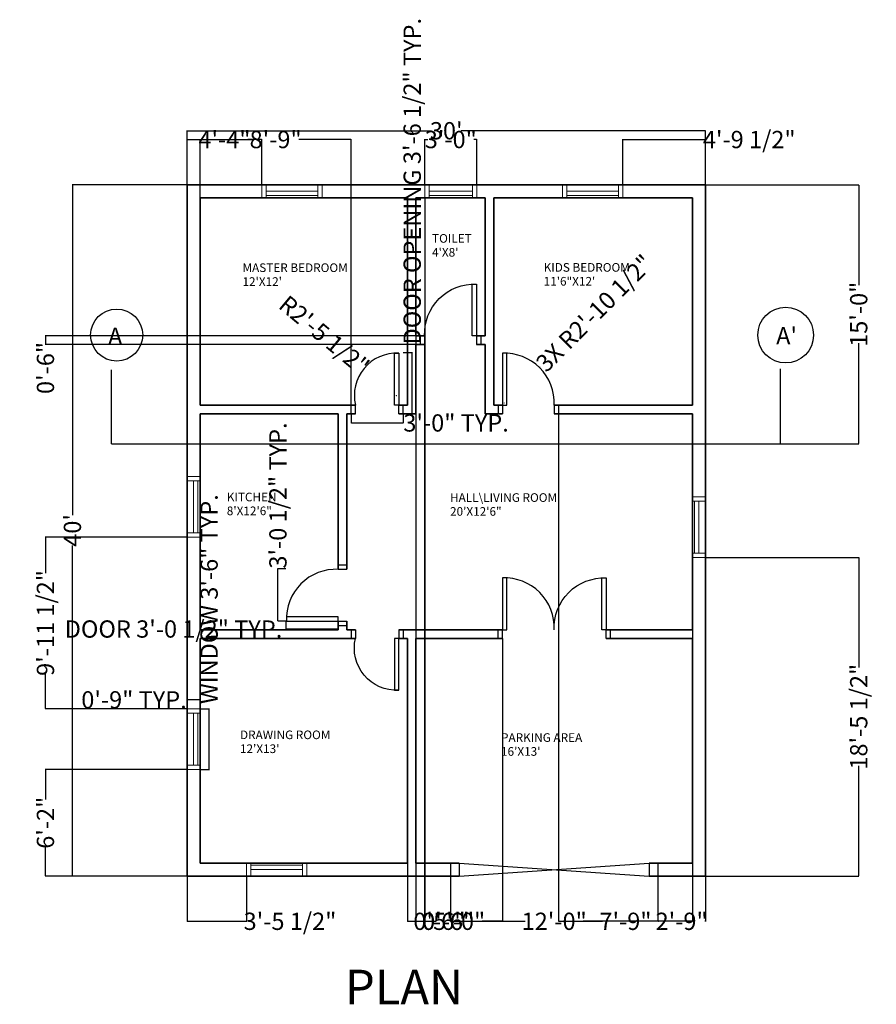
# Model space of a CAD drawing. Units: inches. Extents: x -91 to 1027, y -85 to 599.
# Tile 1 of 3: x -91 to 504, y -85 to 599. Entities that reach past the tile are written whole.
import ezdxf

# ---------------------------------------------------------------- set-up
doc = ezdxf.new("R2010")
doc.units = ezdxf.units.IN
doc.header["$MEASUREMENT"] = 0
for name, color, linetype, lineweight in [('A-ANNO-DIMS', 2, 'Continuous', 18), ('A-ANNO-SYMB', 1, 'Continuous', 25), ('A-ANNO-TEXT', 7, 'Continuous', 35), ('A-AREA-IDEN', 7, 'Continuous', 18), ('A-DOOR', 3, 'Continuous', 25), ('A-DOOR-GATE', 3, 'Continuous', 25), ('A-GLAZ', 4, 'Continuous', 18), ('A-WALL', 7, 'Continuous', 35)]:
    doc.layers.add(name, color=color, linetype=linetype, lineweight=lineweight)
doc.styles.get("Standard").update_dxf_attribs({"font": 'arial.ttf'})
doc.dimstyles.get("Standard").update_dxf_attribs({"dimtxt": 12, "dimasz": 0.18, "dimexe": 0.18, "dimexo": 0.0625, "dimgap": 0.09, "dimtad": 0, "dimdec": 1, "dimzin": 0, "dimdsep": 46, "dimlunit": 3, "dimtxsty": 'Standard', "dimcen": 0.09, "dimadec": 0, "dimazin": 0, "dimtfac": 1, "dimtdec": 1, "dimtofl": 0, "dimtmove": 0, "dimatfit": 3, "dimfxl": 1, "dimtolj": 1, "dimtzin": 0, "dimarcsym": 0})

# ---------------------------------------------------------------- blocks, each defined once
blk = doc.blocks.new('*D1')
at = {"layer": 'A-ANNO-DIMS', "color": 0, "lineweight": -2, "transparency": 16777216}
for p, q in [((25.15, 484.59), (25.15, 522.21)), ((25.33, 522.03), (194.88, 522.03)), ((384.97, 522.03), (215.41, 522.03)), ((385.15, 484.59), (385.15, 522.21))]:
    blk.add_line(p, q, dxfattribs=at)
at = {"layer": 'A-ANNO-DIMS', "color": 0, "transparency": 16777216}
for points in [[(25.33, 522.06), (25.33, 522), (25.15, 522.03)], [(384.97, 522.06), (384.97, 522), (385.15, 522.03)]]:
    blk.add_solid(points, dxfattribs=at)
at = {"layer": 'Defpoints', "color": 0, "transparency": 16777216}
for p in [(385.15, 522.03), (25.15, 484.52), (385.15, 484.52)]:
    blk.add_point(p, dxfattribs=at)
at = {"layer": 'A-ANNO-DIMS', "color": 0, "transparency": 16777216, "insert": (205.15, 522.03), "char_height": 12, "attachment_point": 5}
blk.add_mtext("\\A1;30'", dxfattribs=at)
blk = doc.blocks.new('*D2')
at = {"layer": 'A-ANNO-DIMS', "color": 0, "lineweight": -2, "transparency": 16777216}
for p, q in [((25.08, 484.52), (-54.67, 484.52)), ((-54.49, 484.34), (-54.49, 255.04)), ((-54.49, 4.7), (-54.49, 234.01)), ((25.08, 4.52), (-54.67, 4.52))]:
    blk.add_line(p, q, dxfattribs=at)
at = {"layer": 'A-ANNO-DIMS', "color": 0, "transparency": 16777216}
for points in [[(-54.52, 484.34), (-54.46, 484.34), (-54.49, 484.52)], [(-54.52, 4.7), (-54.46, 4.7), (-54.49, 4.52)]]:
    blk.add_solid(points, dxfattribs=at)
at = {"layer": 'Defpoints', "color": 0, "transparency": 16777216}
for p in [(-54.49, 484.52), (25.15, 484.52), (25.15, 4.52)]:
    blk.add_point(p, dxfattribs=at)
at = {"layer": 'A-ANNO-DIMS', "color": 0, "transparency": 16777216, "insert": (-54.49, 244.52), "char_height": 12, "attachment_point": 5, "rotation": 90}
blk.add_mtext("\\A1;40'", dxfattribs=at)
blk = doc.blocks.new('WIN-36-PLAN')
for p, q in [((0, 9), (0, 0)), ((39, 9), (3, 9)), ((3, 9), (3, 0)), ((39, 0), (39, 9)), ((42, 0), (42, 9)), ((3, 4.5), (39, 4.5)), ((3, 1.5), (39, 1.5)), ((3, 0), (39, 0))]:
    blk.add_line(p, q)
blk = doc.blocks.new('DOOR-36-PLAN')
blk.add_lwpolyline([(0, 0), (3, 0), (3, 36), (0, 36)], close=True)
blk.add_arc((1.5, 1.5), 34.53, 357.51045, 92.48955)
blk = doc.blocks.new('DOOR-30-OPENING-PLAN')
for p, q in [((0, 0), (0, 6)), ((3, 0), (3, 6)), ((33, 0), (33, 6)), ((36, 0), (36, 6))]:
    blk.add_line(p, q)
blk.add_lwpolyline([(33, 6), (30, 6), (30, 42), (33, 42)], close=True)
blk.add_arc((31.5, 12.75), 29.29, 87.06433, 193.32453)
blk = doc.blocks.new('*D24')
at = {"layer": 'A-ANNO-DIMS', "color": 0, "lineweight": -2, "transparency": 16777216}
for p, q in [((34.21, 120.6), (40.63, 120.6)), ((40.45, 120.6), (40.45, 120.78)), ((40.45, 78.78), (40.45, 120.42)), ((34.21, 78.6), (40.63, 78.6))]:
    blk.add_line(p, q, dxfattribs=at)
at = {"layer": 'A-ANNO-DIMS', "color": 0, "transparency": 16777216}
for points in [[(40.42, 120.42), (40.48, 120.42), (40.45, 120.6)], [(40.42, 78.78), (40.48, 78.78), (40.45, 78.6)]]:
    blk.add_solid(points, dxfattribs=at)
at = {"layer": 'Defpoints', "color": 0, "transparency": 16777216}
for p in [(34.15, 120.6), (40.45, 120.6), (34.15, 78.6)]:
    blk.add_point(p, dxfattribs=at)
at = {"layer": 'A-ANNO-DIMS', "color": 0, "transparency": 16777216, "insert": (40.45, 196.8), "char_height": 12, "attachment_point": 5, "rotation": 90}
blk.add_mtext('\\A1;WINDOW 3\'-6" TYP.', dxfattribs=at)
blk = doc.blocks.new('*D25')
at = {"layer": 'A-ANNO-DIMS', "color": 0, "lineweight": -2, "transparency": 16777216}
for p, q in [((25.15, 126.9), (24.97, 126.9)), ((25.15, 120.67), (25.15, 127.08)), ((33.97, 126.9), (25.33, 126.9)), ((34.15, 120.67), (34.15, 127.08))]:
    blk.add_line(p, q, dxfattribs=at)
at = {"layer": 'A-ANNO-DIMS', "color": 0, "transparency": 16777216}
for points in [[(25.33, 126.93), (25.33, 126.87), (25.15, 126.9)], [(33.97, 126.93), (33.97, 126.87), (34.15, 126.9)]]:
    blk.add_solid(points, dxfattribs=at)
at = {"layer": 'Defpoints', "color": 0, "transparency": 16777216}
for p in [(25.15, 126.9), (25.15, 120.6), (34.15, 120.6)]:
    blk.add_point(p, dxfattribs=at)
at = {"layer": 'A-ANNO-DIMS', "color": 0, "transparency": 16777216, "insert": (-11.7, 126.9), "char_height": 12, "attachment_point": 5}
blk.add_mtext('\\A1;0\'-9" TYP.', dxfattribs=at)
blk = doc.blocks.new('*D26')
at = {"layer": 'A-ANNO-DIMS', "color": 0, "lineweight": -2, "transparency": 16777216}
for p, q in [((93.73, 181.46), (93.73, 175.88)), ((130.15, 181.46), (130.15, 175.88)), ((93.73, 176.06), (93.55, 176.06)), ((129.97, 176.06), (93.91, 176.06))]:
    blk.add_line(p, q, dxfattribs=at)
at = {"layer": 'A-ANNO-DIMS', "color": 0, "transparency": 16777216}
for points in [[(93.91, 176.09), (93.91, 176.03), (93.73, 176.06)], [(129.97, 176.09), (129.97, 176.03), (130.15, 176.06)]]:
    blk.add_solid(points, dxfattribs=at)
at = {"layer": 'Defpoints', "color": 0, "transparency": 16777216}
for p in [(93.73, 181.52), (130.15, 181.52), (93.73, 176.06)]:
    blk.add_point(p, dxfattribs=at)
at = {"layer": 'A-ANNO-DIMS', "color": 0, "transparency": 16777216, "insert": (15.73, 176.06), "char_height": 12, "attachment_point": 5}
blk.add_mtext('\\A1;DOOR 3\'-0 1/2" TYP.', dxfattribs=at)
blk = doc.blocks.new('*D27')
at = {"layer": 'A-ANNO-DIMS', "color": 0, "lineweight": -2, "transparency": 16777216}
for p, q in [((93.66, 217.94), (88.08, 217.94)), ((88.26, 217.94), (88.26, 218.12)), ((88.26, 181.7), (88.26, 217.76)), ((93.66, 181.52), (88.08, 181.52))]:
    blk.add_line(p, q, dxfattribs=at)
at = {"layer": 'A-ANNO-DIMS', "color": 0, "transparency": 16777216}
for points in [[(88.23, 217.76), (88.29, 217.76), (88.26, 217.94)], [(88.23, 181.7), (88.29, 181.7), (88.26, 181.52)]]:
    blk.add_solid(points, dxfattribs=at)
at = {"layer": 'Defpoints', "color": 0, "transparency": 16777216}
for p in [(88.26, 217.94), (93.73, 217.94), (93.73, 181.52)]:
    blk.add_point(p, dxfattribs=at)
at = {"layer": 'A-ANNO-DIMS', "color": 0, "transparency": 16777216, "insert": (88.26, 268.76), "char_height": 12, "attachment_point": 5, "rotation": 90}
blk.add_mtext('\\A1;3\'-0 1/2" TYP.', dxfattribs=at)
blk = doc.blocks.new('*D28')
at = {"layer": 'A-ANNO-DIMS', "color": 0, "lineweight": -2, "transparency": 16777216}
for p, q in [((175.21, 368), (181.7, 368)), ((181.52, 368), (181.52, 368.18)), ((181.52, 325.7), (181.52, 367.82)), ((175.21, 325.52), (181.7, 325.52))]:
    blk.add_line(p, q, dxfattribs=at)
at = {"layer": 'A-ANNO-DIMS', "color": 0, "transparency": 16777216}
for points in [[(181.49, 367.82), (181.55, 367.82), (181.52, 368)], [(181.49, 325.7), (181.55, 325.7), (181.52, 325.52)]]:
    blk.add_solid(points, dxfattribs=at)
at = {"layer": 'Defpoints', "color": 0, "transparency": 16777216}
for p in [(175.15, 368), (181.52, 368), (175.15, 325.52)]:
    blk.add_point(p, dxfattribs=at)
at = {"layer": 'A-ANNO-DIMS', "color": 0, "transparency": 16777216, "insert": (181.52, 486.98), "char_height": 12, "attachment_point": 5, "rotation": 90}
blk.add_mtext('\\A1;DOOR OPENING 3\'-6 1/2" TYP.', dxfattribs=at)
blk = doc.blocks.new('*D29')
at = {"layer": 'A-ANNO-DIMS', "color": 0, "lineweight": -2, "transparency": 16777216}
for p, q in [((139.15, 325.46), (139.15, 318.97)), ((175.15, 325.46), (175.15, 318.97)), ((139.33, 319.15), (174.97, 319.15)), ((175.15, 319.15), (175.33, 319.15))]:
    blk.add_line(p, q, dxfattribs=at)
at = {"layer": 'A-ANNO-DIMS', "color": 0, "transparency": 16777216}
for points in [[(139.33, 319.18), (139.33, 319.12), (139.15, 319.15)], [(174.97, 319.18), (174.97, 319.12), (175.15, 319.15)]]:
    blk.add_solid(points, dxfattribs=at)
at = {"layer": 'Defpoints', "color": 0, "transparency": 16777216}
for p in [(139.15, 325.52), (175.15, 325.52), (175.15, 319.15)]:
    blk.add_point(p, dxfattribs=at)
at = {"layer": 'A-ANNO-DIMS', "color": 0, "transparency": 16777216, "insert": (211.98, 319.15), "char_height": 12, "attachment_point": 5}
blk.add_mtext('\\A1;3\'-0" TYP.', dxfattribs=at)
blk = doc.blocks.new('*D36')
at = {"layer": 'A-ANNO-DIMS', "color": 0, "lineweight": -2, "transparency": 16777216}
for p, q in [((25.15, 484.59), (25.15, 516.1)), ((25.33, 515.92), (34.83, 515.92)), ((76.89, 515.92), (67.39, 515.92)), ((77.07, 484.59), (77.07, 516.1))]:
    blk.add_line(p, q, dxfattribs=at)
at = {"layer": 'A-ANNO-DIMS', "color": 0, "transparency": 16777216}
for points in [[(25.33, 515.95), (25.33, 515.89), (25.15, 515.92)], [(76.89, 515.95), (76.89, 515.89), (77.07, 515.92)]]:
    blk.add_solid(points, dxfattribs=at)
at = {"layer": 'Defpoints', "color": 0, "transparency": 16777216}
for p in [(77.07, 515.92), (25.15, 484.52), (77.07, 484.52)]:
    blk.add_point(p, dxfattribs=at)
at = {"layer": 'A-ANNO-DIMS', "color": 0, "transparency": 16777216, "insert": (51.11, 515.92), "char_height": 12, "attachment_point": 5}
blk.add_mtext('\\A1;4\'-4"', dxfattribs=at)
blk = doc.blocks.new('*D37')
at = {"layer": 'A-ANNO-DIMS', "color": 0, "lineweight": -2, "transparency": 16777216}
for p, q in [((184.15, 475.46), (184.15, -27.06)), ((190.32, 475.46), (190.32, -27.06)), ((184.33, -26.88), (190.14, -26.88)), ((190.32, -26.88), (190.5, -26.88))]:
    blk.add_line(p, q, dxfattribs=at)
at = {"layer": 'A-ANNO-DIMS', "color": 0, "transparency": 16777216}
for points in [[(184.33, -26.85), (184.33, -26.91), (184.15, -26.88)], [(190.14, -26.85), (190.14, -26.91), (190.32, -26.88)]]:
    blk.add_solid(points, dxfattribs=at)
at = {"layer": 'Defpoints', "color": 0, "transparency": 16777216}
for p in [(184.15, 475.52), (190.32, 475.52), (190.32, -26.88)]:
    blk.add_point(p, dxfattribs=at)
at = {"layer": 'A-ANNO-DIMS', "color": 0, "transparency": 16777216, "insert": (206.54, -26.88), "char_height": 12, "attachment_point": 5}
blk.add_mtext('\\A1;0\'-6"', dxfattribs=at)
blk = doc.blocks.new('*D38')
at = {"layer": 'A-ANNO-DIMS', "color": 0, "lineweight": -2, "transparency": 16777216}
for p, q in [((190.32, 484.59), (190.32, 516.1)), ((190.5, 515.92), (192.29, 515.92)), ((226.14, 515.92), (224.36, 515.92)), ((226.32, 484.59), (226.32, 516.1))]:
    blk.add_line(p, q, dxfattribs=at)
at = {"layer": 'A-ANNO-DIMS', "color": 0, "transparency": 16777216}
for points in [[(190.5, 515.95), (190.5, 515.89), (190.32, 515.92)], [(226.14, 515.95), (226.14, 515.89), (226.32, 515.92)]]:
    blk.add_solid(points, dxfattribs=at)
at = {"layer": 'Defpoints', "color": 0, "transparency": 16777216}
for p in [(226.32, 515.92), (190.32, 484.52), (226.32, 484.52)]:
    blk.add_point(p, dxfattribs=at)
at = {"layer": 'A-ANNO-DIMS', "color": 0, "transparency": 16777216, "insert": (208.32, 515.92), "char_height": 12, "attachment_point": 5}
blk.add_mtext('\\A1;3\'-0"', dxfattribs=at)
blk = doc.blocks.new('*D39')
at = {"layer": 'A-ANNO-DIMS', "color": 0, "lineweight": -2, "transparency": 16777216}
for p, q in [((327.88, 484.59), (327.88, 516.1)), ((328.06, 515.92), (384.97, 515.92)), ((385.15, 484.59), (385.15, 516.1)), ((385.15, 515.92), (385.33, 515.92))]:
    blk.add_line(p, q, dxfattribs=at)
at = {"layer": 'A-ANNO-DIMS', "color": 0, "transparency": 16777216}
for points in [[(328.06, 515.95), (328.06, 515.89), (327.88, 515.92)], [(384.97, 515.95), (384.97, 515.89), (385.15, 515.92)]]:
    blk.add_solid(points, dxfattribs=at)
at = {"layer": 'Defpoints', "color": 0, "transparency": 16777216}
for p in [(385.15, 515.92), (327.88, 484.52), (385.15, 484.52)]:
    blk.add_point(p, dxfattribs=at)
at = {"layer": 'A-ANNO-DIMS', "color": 0, "transparency": 16777216, "insert": (415.59, 515.92), "char_height": 12, "attachment_point": 5}
blk.add_mtext('\\A1;4\'-9 1/2"', dxfattribs=at)
blk = doc.blocks.new('*D40')
at = {"layer": 'A-ANNO-DIMS', "color": 0, "lineweight": -2, "transparency": 16777216}
for p, q in [((25.15, 4.46), (25.15, -27.06)), ((66.43, 4.46), (66.43, -27.06)), ((25.33, -26.88), (66.25, -26.88)), ((66.43, -26.88), (66.61, -26.88))]:
    blk.add_line(p, q, dxfattribs=at)
at = {"layer": 'A-ANNO-DIMS', "color": 0, "transparency": 16777216}
for points in [[(25.33, -26.85), (25.33, -26.91), (25.15, -26.88)], [(66.25, -26.85), (66.25, -26.91), (66.43, -26.88)]]:
    blk.add_solid(points, dxfattribs=at)
at = {"layer": 'Defpoints', "color": 0, "transparency": 16777216}
for p in [(25.15, 4.52), (66.43, 4.52), (66.43, -26.88)]:
    blk.add_point(p, dxfattribs=at)
at = {"layer": 'A-ANNO-DIMS', "color": 0, "transparency": 16777216, "insert": (96.63, -26.88), "char_height": 12, "attachment_point": 5}
blk.add_mtext('\\A1;3\'-5 1/2"', dxfattribs=at)
blk = doc.blocks.new('*D41')
at = {"layer": 'A-ANNO-DIMS', "color": 0, "lineweight": -2, "transparency": 16777216}
for p, q in [((352.15, 4.46), (352.15, -27.06)), ((385.15, 4.46), (385.15, -27.06)), ((352.33, -26.88), (352.5, -26.88)), ((384.97, -26.88), (384.79, -26.88))]:
    blk.add_line(p, q, dxfattribs=at)
at = {"layer": 'A-ANNO-DIMS', "color": 0, "transparency": 16777216}
for points in [[(352.33, -26.85), (352.33, -26.91), (352.15, -26.88)], [(384.97, -26.85), (384.97, -26.91), (385.15, -26.88)]]:
    blk.add_solid(points, dxfattribs=at)
at = {"layer": 'Defpoints', "color": 0, "transparency": 16777216}
for p in [(352.15, 4.52), (385.15, 4.52), (352.15, -26.88)]:
    blk.add_point(p, dxfattribs=at)
at = {"layer": 'A-ANNO-DIMS', "color": 0, "transparency": 16777216, "insert": (368.65, -26.88), "char_height": 12, "attachment_point": 5}
blk.add_mtext('\\A1;2\'-9"', dxfattribs=at)
blk = doc.blocks.new('*D42')
at = {"layer": 'A-ANNO-DIMS', "color": 0, "lineweight": -2, "transparency": 16777216}
for p, q in [((208.15, 4.46), (208.15, -27.06)), ((352.15, 4.46), (352.15, -27.06)), ((208.33, -26.88), (260.01, -26.88)), ((351.97, -26.88), (300.28, -26.88))]:
    blk.add_line(p, q, dxfattribs=at)
at = {"layer": 'A-ANNO-DIMS', "color": 0, "transparency": 16777216}
for points in [[(208.33, -26.85), (208.33, -26.91), (208.15, -26.88)], [(351.97, -26.85), (351.97, -26.91), (352.15, -26.88)]]:
    blk.add_solid(points, dxfattribs=at)
at = {"layer": 'Defpoints', "color": 0, "transparency": 16777216}
for p in [(208.15, 4.52), (352.15, 4.52), (352.15, -26.88)]:
    blk.add_point(p, dxfattribs=at)
at = {"layer": 'A-ANNO-DIMS', "color": 0, "transparency": 16777216, "insert": (280.15, -26.88), "char_height": 12, "attachment_point": 5}
blk.add_mtext('\\A1;12\'-0"', dxfattribs=at)
blk = doc.blocks.new('*D43')
at = {"layer": 'A-ANNO-DIMS', "color": 0, "lineweight": -2, "transparency": 16777216}
for p, q in [((25.08, 78.6), (-73.39, 78.6)), ((-73.21, 78.42), (-73.21, 57.64)), ((-73.21, 4.7), (-73.21, 25.49)), ((25.08, 4.52), (-73.39, 4.52))]:
    blk.add_line(p, q, dxfattribs=at)
at = {"layer": 'A-ANNO-DIMS', "color": 0, "transparency": 16777216}
for points in [[(-73.24, 78.42), (-73.18, 78.42), (-73.21, 78.6)], [(-73.24, 4.7), (-73.18, 4.7), (-73.21, 4.52)]]:
    blk.add_solid(points, dxfattribs=at)
at = {"layer": 'Defpoints', "color": 0, "transparency": 16777216}
for p in [(-73.21, 78.6), (25.15, 78.6), (25.15, 4.52)]:
    blk.add_point(p, dxfattribs=at)
at = {"layer": 'A-ANNO-DIMS', "color": 0, "transparency": 16777216, "insert": (-73.21, 41.56), "char_height": 12, "attachment_point": 5, "rotation": 90}
blk.add_mtext('\\A1;6\'-2"', dxfattribs=at)
blk = doc.blocks.new('*D44')
at = {"layer": 'A-ANNO-DIMS', "color": 0, "lineweight": -2, "transparency": 16777216}
for p, q in [((25.08, 239.92), (-73.39, 239.92)), ((-73.21, 239.74), (-73.21, 214.95)), ((-73.21, 120.78), (-73.21, 145.58)), ((25.08, 120.6), (-73.39, 120.6))]:
    blk.add_line(p, q, dxfattribs=at)
at = {"layer": 'A-ANNO-DIMS', "color": 0, "transparency": 16777216}
for points in [[(-73.24, 239.74), (-73.18, 239.74), (-73.21, 239.92)], [(-73.24, 120.78), (-73.18, 120.78), (-73.21, 120.6)]]:
    blk.add_solid(points, dxfattribs=at)
at = {"layer": 'Defpoints', "color": 0, "transparency": 16777216}
for p in [(25.15, 239.92), (-73.21, 120.6), (25.15, 120.6)]:
    blk.add_point(p, dxfattribs=at)
at = {"layer": 'A-ANNO-DIMS', "color": 0, "transparency": 16777216, "insert": (-73.21, 180.26), "char_height": 12, "attachment_point": 5, "rotation": 90}
blk.add_mtext('\\A1;9\'-11 1/2"', dxfattribs=at)
blk = doc.blocks.new('*D45')
at = {"layer": 'A-ANNO-DIMS', "color": 0, "lineweight": -2, "transparency": 16777216}
for p, q in [((385.21, 225.81), (491.83, 225.81)), ((491.65, 225.63), (491.65, 149.28)), ((491.65, 4.7), (491.65, 81.05)), ((385.21, 4.52), (491.83, 4.52))]:
    blk.add_line(p, q, dxfattribs=at)
at = {"layer": 'A-ANNO-DIMS', "color": 0, "transparency": 16777216}
for points in [[(491.62, 225.63), (491.68, 225.63), (491.65, 225.81)], [(491.62, 4.7), (491.68, 4.7), (491.65, 4.52)]]:
    blk.add_solid(points, dxfattribs=at)
at = {"layer": 'Defpoints', "color": 0, "transparency": 16777216}
for p in [(385.15, 225.81), (491.65, 225.81), (385.15, 4.52)]:
    blk.add_point(p, dxfattribs=at)
at = {"layer": 'A-ANNO-DIMS', "color": 0, "transparency": 16777216, "insert": (491.65, 115.17), "char_height": 12, "attachment_point": 5, "rotation": 90}
blk.add_mtext('\\A1;18\'-5 1/2"', dxfattribs=at)
blk = doc.blocks.new('*D46')
at = {"layer": 'A-ANNO-DIMS', "color": 0, "lineweight": -2, "transparency": 16777216}
for p, q in [((178.15, 13.46), (178.15, -27.06)), ((184.15, 13.46), (184.15, -27.06)), ((178.33, -26.88), (183.97, -26.88)), ((184.15, -26.88), (184.33, -26.88))]:
    blk.add_line(p, q, dxfattribs=at)
at = {"layer": 'A-ANNO-DIMS', "color": 0, "transparency": 16777216}
for points in [[(178.33, -26.85), (178.33, -26.91), (178.15, -26.88)], [(183.97, -26.85), (183.97, -26.91), (184.15, -26.88)]]:
    blk.add_solid(points, dxfattribs=at)
at = {"layer": 'Defpoints', "color": 0, "transparency": 16777216}
for p in [(178.15, 13.52), (184.15, 13.52), (184.15, -26.88)]:
    blk.add_point(p, dxfattribs=at)
at = {"layer": 'A-ANNO-DIMS', "color": 0, "transparency": 16777216, "insert": (200.37, -26.88), "char_height": 12, "attachment_point": 5}
blk.add_mtext('\\A1;0\'-6"', dxfattribs=at)
blk = doc.blocks.new('*D47')
at = {"layer": 'A-ANNO-DIMS', "color": 0, "lineweight": -2, "transparency": 16777216}
for p, q in [((385.21, 484.52), (491.83, 484.52)), ((491.65, 484.34), (491.65, 414.74)), ((491.65, 304.87), (491.65, 374.47)), ((437.43, 304.69), (491.83, 304.69))]:
    blk.add_line(p, q, dxfattribs=at)
at = {"layer": 'A-ANNO-DIMS', "color": 0, "transparency": 16777216}
for points in [[(491.62, 484.34), (491.68, 484.34), (491.65, 484.52)], [(491.62, 304.87), (491.68, 304.87), (491.65, 304.69)]]:
    blk.add_solid(points, dxfattribs=at)
at = {"layer": 'Defpoints', "color": 0, "transparency": 16777216}
for p in [(385.15, 484.52), (491.65, 484.52), (437.37, 304.69)]:
    blk.add_point(p, dxfattribs=at)
at = {"layer": 'A-ANNO-DIMS', "color": 0, "transparency": 16777216, "insert": (491.65, 394.6), "char_height": 12, "attachment_point": 5, "rotation": 90}
blk.add_mtext('\\A1;15\'-0"', dxfattribs=at)
blk = doc.blocks.new('*D48')
at = {"layer": 'A-ANNO-DIMS', "color": 0, "lineweight": -2, "transparency": 16777216}
for p, q in [((184.15, 169.46), (184.15, -27.06)), ((244.15, 169.46), (244.15, -27.06)), ((184.33, -26.88), (198.11, -26.88)), ((243.97, -26.88), (230.19, -26.88))]:
    blk.add_line(p, q, dxfattribs=at)
at = {"layer": 'A-ANNO-DIMS', "color": 0, "transparency": 16777216}
for points in [[(184.33, -26.85), (184.33, -26.91), (184.15, -26.88)], [(243.97, -26.85), (243.97, -26.91), (244.15, -26.88)]]:
    blk.add_solid(points, dxfattribs=at)
at = {"layer": 'Defpoints', "color": 0, "transparency": 16777216}
for p in [(184.15, 169.52), (244.15, 169.52), (244.15, -26.88)]:
    blk.add_point(p, dxfattribs=at)
at = {"layer": 'A-ANNO-DIMS', "color": 0, "transparency": 16777216, "insert": (214.15, -26.88), "char_height": 12, "attachment_point": 5}
blk.add_mtext('\\A1;5\'-0"', dxfattribs=at)
blk = doc.blocks.new('*D49')
at = {"layer": 'A-ANNO-DIMS', "color": 0, "lineweight": -2, "transparency": 16777216}
for p, q in [((283.15, 325.46), (283.15, -27.06)), ((376.15, 325.46), (376.15, -27.06)), ((283.33, -26.88), (313.66, -26.88)), ((375.97, -26.88), (345.64, -26.88))]:
    blk.add_line(p, q, dxfattribs=at)
at = {"layer": 'A-ANNO-DIMS', "color": 0, "transparency": 16777216}
for points in [[(283.33, -26.85), (283.33, -26.91), (283.15, -26.88)], [(375.97, -26.85), (375.97, -26.91), (376.15, -26.88)]]:
    blk.add_solid(points, dxfattribs=at)
at = {"layer": 'Defpoints', "color": 0, "transparency": 16777216}
for p in [(283.15, 325.52), (376.15, 325.52), (376.15, -26.88)]:
    blk.add_point(p, dxfattribs=at)
at = {"layer": 'A-ANNO-DIMS', "color": 0, "transparency": 16777216, "insert": (329.65, -26.88), "char_height": 12, "attachment_point": 5}
blk.add_mtext('\\A1;7\'-9"', dxfattribs=at)
blk = doc.blocks.new('*D50')
at = {"layer": 'A-ANNO-DIMS', "color": 0, "lineweight": -2, "transparency": 16777216}
for p, q in [((184.15, 379.46), (184.15, -27.06)), ((190.15, 379.46), (190.15, -27.06)), ((184.33, -26.88), (189.97, -26.88)), ((190.15, -26.88), (190.33, -26.88))]:
    blk.add_line(p, q, dxfattribs=at)
at = {"layer": 'A-ANNO-DIMS', "color": 0, "transparency": 16777216}
for points in [[(184.33, -26.85), (184.33, -26.91), (184.15, -26.88)], [(189.97, -26.85), (189.97, -26.91), (190.15, -26.88)]]:
    blk.add_solid(points, dxfattribs=at)
at = {"layer": 'Defpoints', "color": 0, "transparency": 16777216}
for p in [(184.15, 379.52), (190.15, 379.52), (190.15, -26.88)]:
    blk.add_point(p, dxfattribs=at)
at = {"layer": 'A-ANNO-DIMS', "color": 0, "transparency": 16777216, "insert": (206.37, -26.88), "char_height": 12, "attachment_point": 5}
blk.add_mtext('\\A1;0\'-6"', dxfattribs=at)
blk = doc.blocks.new('*D51')
at = {"layer": 'A-ANNO-DIMS', "color": 0, "lineweight": -2, "transparency": 16777216}
for p, q in [((184.08, 379.52), (-73.39, 379.52)), ((-73.21, 379.34), (-73.21, 373.7)), ((184.08, 373.52), (-73.39, 373.52)), ((-73.21, 373.52), (-73.21, 373.34))]:
    blk.add_line(p, q, dxfattribs=at)
at = {"layer": 'A-ANNO-DIMS', "color": 0, "transparency": 16777216}
for points in [[(-73.24, 379.34), (-73.18, 379.34), (-73.21, 379.52)], [(-73.24, 373.7), (-73.18, 373.7), (-73.21, 373.52)]]:
    blk.add_solid(points, dxfattribs=at)
at = {"layer": 'Defpoints', "color": 0, "transparency": 16777216}
for p in [(184.15, 379.52), (-73.21, 373.52), (184.15, 373.52)]:
    blk.add_point(p, dxfattribs=at)
at = {"layer": 'A-ANNO-DIMS', "color": 0, "transparency": 16777216, "insert": (-73.21, 357.3), "char_height": 12, "attachment_point": 5, "rotation": 90}
blk.add_mtext('\\A1;0\'-6"', dxfattribs=at)
blk = doc.blocks.new('*D52')
at = {"layer": 'A-ANNO-DIMS', "color": 0, "lineweight": -2, "transparency": 16777216}
for p, q in [((34.15, 331.59), (34.15, 516.1)), ((34.33, 515.92), (70.6, 515.92)), ((138.97, 515.92), (102.69, 515.92)), ((139.15, 331.59), (139.15, 516.1))]:
    blk.add_line(p, q, dxfattribs=at)
at = {"layer": 'A-ANNO-DIMS', "color": 0, "transparency": 16777216}
for points in [[(34.33, 515.95), (34.33, 515.89), (34.15, 515.92)], [(138.97, 515.95), (138.97, 515.89), (139.15, 515.92)]]:
    blk.add_solid(points, dxfattribs=at)
at = {"layer": 'Defpoints', "color": 0, "transparency": 16777216}
for p in [(139.15, 515.92), (34.15, 331.52), (139.15, 331.52)]:
    blk.add_point(p, dxfattribs=at)
at = {"layer": 'A-ANNO-DIMS', "color": 0, "transparency": 16777216, "insert": (86.65, 515.92), "char_height": 12, "attachment_point": 5}
blk.add_mtext('\\A1;8\'-9"', dxfattribs=at)
blk = doc.blocks.new('*D68')
at = {"layer": 'A-ANNO-DIMS', "color": 0, "lineweight": -2, "transparency": 16777216}
for p, q in [((270.32, 357.7), (270.19, 357.57)), ((245.56, 333.02), (245.74, 333.02)), ((245.65, 332.93), (245.65, 333.11))]:
    blk.add_line(p, q, dxfattribs=at)
at = {"layer": 'A-ANNO-DIMS', "color": 0, "transparency": 16777216}
blk.add_solid([(270.17, 357.59), (270.21, 357.55), (270.06, 357.44)], dxfattribs=at)
at = {"layer": 'Defpoints', "color": 0, "transparency": 16777216}
for p in [(270.06, 357.44), (245.65, 333.02)]:
    blk.add_point(p, dxfattribs=at)
at = {"layer": 'A-ANNO-DIMS', "color": 0, "transparency": 16777216, "insert": (308.02, 395.39), "char_height": 12, "attachment_point": 5, "rotation": 44.99999}
blk.add_mtext('\\A1;3X R2\'-10 1/2"', dxfattribs=at)
blk = doc.blocks.new('*D69')
at = {"layer": 'A-ANNO-DIMS', "color": 0, "lineweight": -2, "transparency": 16777216}
for p, q in [((147.87, 357.25), (148.01, 357.14)), ((170.56, 338.27), (170.74, 338.27)), ((170.65, 338.18), (170.65, 338.36))]:
    blk.add_line(p, q, dxfattribs=at)
at = {"layer": 'A-ANNO-DIMS', "color": 0, "transparency": 16777216}
blk.add_solid([(148.03, 357.16), (147.99, 357.12), (148.15, 357.02)], dxfattribs=at)
at = {"layer": 'Defpoints', "color": 0, "transparency": 16777216}
for p in [(148.15, 357.02), (170.65, 338.27)]:
    blk.add_point(p, dxfattribs=at)
at = {"layer": 'A-ANNO-DIMS', "color": 0, "transparency": 16777216, "insert": (120.4, 380.15), "char_height": 12, "attachment_point": 5, "rotation": 320.19311}
blk.add_mtext('\\A1;R2\'-5 1/2"', dxfattribs=at)

msp = doc.modelspace()

# ---------------------------------------------------------------- linework, layer by layer
at = {"layer": 'A-ANNO-SYMB'}
for p, q in [((-27.4, 304.69), (-27.4, 355.99)), ((437.37, 329.85), (437.37, 356.64)), ((437.37, 304.69), (437.37, 329.85)), ((-27.4, 304.69), (437.37, 304.69))]:
    msp.add_line(p, q, dxfattribs=at)
for centre, radius in [((-23.74, 380.17), 18.07), ((440.9, 380.15), 19.36)]:
    msp.add_circle(centre, radius, dxfattribs=at)
at = {"layer": 'A-DOOR'}
for p, q in [((187.15, 379.52), (187.15, 373.52)), ((190.15, 379.52), (190.15, 373.52)), ((226.15, 379.52), (226.15, 373.52)), ((229.15, 379.52), (229.15, 373.52)), ((241.15, 331.52), (241.15, 325.52)), ((244.15, 331.52), (244.15, 325.52)), ((280.15, 331.52), (280.15, 325.52)), ((283.15, 331.52), (283.15, 325.52)), ((130.15, 220.52), (136.15, 220.52)), ((130.15, 217.52), (136.15, 217.52)), ((130.15, 181.52), (136.15, 181.52)), ((130.15, 178.52), (136.15, 178.52)), ((241.15, 169.52), (241.15, 175.52)), ((244.15, 169.52), (244.15, 175.52)), ((316.15, 169.52), (316.15, 175.52)), ((319.15, 169.52), (319.15, 175.52))]:
    msp.add_line(p, q, dxfattribs=at)
at = {"layer": 'A-DOOR-GATE'}
for p, q in [((208.15, 13.52), (208.15, 4.52)), ((214.15, 13.52), (214.15, 4.52)), ((214.15, 13.52), (346.15, 4.52)), ((214.15, 4.52), (346.15, 13.52)), ((346.15, 13.52), (346.15, 4.52)), ((352.15, 13.52), (352.15, 4.52))]:
    msp.add_line(p, q, dxfattribs=at)
at = {"layer": 'A-GLAZ'}
for p, q in [((190.32, 484.52), (190.32, 475.52)), ((223.32, 484.52), (193.32, 484.52)), ((193.32, 484.52), (193.32, 475.52)), ((193.32, 480.02), (223.32, 480.02)), ((223.32, 475.52), (223.32, 484.52)), ((226.32, 475.52), (226.32, 484.52)), ((193.32, 477.02), (223.32, 477.02)), ((193.32, 475.52), (223.32, 475.52))]:
    msp.add_line(p, q, dxfattribs=at)
at = {"layer": 'A-WALL'}
for p, q in [((34.15, 475.52), (34.15, 331.52)), ((178.15, 475.52), (34.15, 475.52)), ((178.15, 475.52), (178.15, 331.52)), ((184.15, 475.52), (184.15, 379.52)), ((232.15, 475.52), (184.15, 475.52)), ((232.15, 475.52), (232.15, 379.52)), ((376.15, 475.52), (238.15, 475.52)), ((238.15, 475.52), (238.15, 331.52)), ((376.15, 331.52), (376.15, 475.52)), ((190.15, 379.52), (184.15, 379.52)), ((232.15, 379.52), (226.15, 379.52)), ((184.15, 373.52), (184.15, 325.52)), ((190.15, 373.52), (184.15, 373.52)), ((232.15, 373.52), (226.15, 373.52)), ((232.15, 373.52), (232.15, 325.52)), ((142.15, 331.52), (34.15, 331.52)), ((178.15, 331.52), (172.15, 331.52)), ((244.15, 331.52), (238.15, 331.52)), ((376.15, 331.52), (280.15, 331.52)), ((34.15, 325.52), (34.15, 175.52)), ((130.15, 325.52), (34.15, 325.52)), ((130.15, 325.52), (130.15, 217.52)), ((136.15, 325.52), (136.15, 217.52)), ((142.15, 325.52), (136.15, 325.52)), ((184.15, 325.52), (172.15, 325.52)), ((178.15, 325.52), (175.15, 325.52)), ((244.15, 325.52), (232.15, 325.52)), ((376.15, 325.52), (280.15, 325.52)), ((376.15, 175.52), (376.15, 325.52)), ((130.15, 181.52), (130.15, 175.52)), ((136.15, 181.52), (136.15, 175.52)), ((130.15, 175.52), (34.15, 175.52)), ((142.15, 175.52), (136.15, 175.52)), ((244.15, 175.52), (172.15, 175.52)), ((376.15, 175.52), (316.15, 175.52)), ((34.15, 169.52), (34.15, 13.52)), ((142.15, 169.52), (34.15, 169.52)), ((178.15, 169.52), (172.15, 169.52)), ((178.15, 169.52), (178.15, 13.52)), ((184.15, 169.52), (184.15, 13.52)), ((244.15, 169.52), (184.15, 169.52)), ((376.15, 169.52), (316.15, 169.52)), ((376.15, 13.52), (376.15, 169.52)), ((34.15, 13.52), (178.15, 13.52)), ((184.15, 13.52), (214.15, 13.52)), ((346.15, 13.52), (376.15, 13.52)), ((376.15, 13.52), (373.15, 13.52))]:
    msp.add_line(p, q, dxfattribs=at)
msp.add_lwpolyline([(346.15, 4.52), (385.15, 4.52), (385.15, 484.52), (25.15, 484.52), (25.15, 4.52), (214.15, 4.52)], dxfattribs=at)

# ---------------------------------------------------------------- block references
at = {"layer": 'A-DOOR', "extrusion": (0, 0, -1), "zscale": -1}
for p in [(-226.15, 379.52), (-316.17, 175.52)]:
    msp.add_blockref('DOOR-36-PLAN', p, dxfattribs=at)
at = {"layer": 'A-DOOR'}
for name, p in [('DOOR-30-OPENING-PLAN', (139.15, 325.52)), ('DOOR-36-PLAN', (244.15, 331.52)), ('DOOR-36-PLAN', (244.15, 175.52))]:
    msp.add_blockref(name, p, dxfattribs=at)
at = {"layer": 'A-DOOR', "rotation": 89.99999999999984}
msp.add_blockref('DOOR-36-PLAN', (130.15, 181.52), dxfattribs=at)
at = {"layer": 'A-DOOR', "extrusion": (0, 0, -1), "zscale": -1, "rotation": 180}
msp.add_blockref('DOOR-30-OPENING-PLAN', (-139.15, 175.52), dxfattribs=at)
at = {"layer": 'A-GLAZ'}
for p in [(77.07, 475.52), (285.88, 475.52)]:
    msp.add_blockref('WIN-36-PLAN', p, dxfattribs=at)
for p, rotation in [((34.15, 239.92), 90), ((376.15, 267.81), 270.0000000000003), ((34.15, 78.6), 90.00000000000006), ((108.43, 13.52), 180)]:
    msp.add_blockref('WIN-36-PLAN', p, dxfattribs=dict(at, rotation=rotation))

# ---------------------------------------------------------------- texts
at = {"layer": 'A-ANNO-SYMB'}
for s, p in [('A', (-29.73, 373.34)), ("A'", (434.28, 373.7))]:
    msp.add_text(s, height=12, dxfattribs=at).set_placement(p)
at = {"layer": 'A-ANNO-TEXT'}
msp.add_text('PLAN', height=24, dxfattribs=at).set_placement((134.81, -84.51))
at = {"layer": 'A-AREA-IDEN'}
for s, p in [('TOILET', (195.32, 444.27)), ("4'X8'", (195.32, 434.63)), ('MASTER BEDROOM', (63.65, 423.94)), ('KIDS BEDROOM', (272.83, 424.14)), ("12'X12'", (63.65, 414.3)), ('11\'6"X12\'', (272.83, 414.5)), ('KITCHEN', (52.76, 264.72)), ('HALL\\LIVING ROOM', (207.79, 264.34)), ('8\'X12\'6"', (52.76, 255.09)), ('20\'X12\'6"', (207.79, 254.7)), ('DRAWING ROOM', (61.91, 99.59)), ('PARKING AREA', (243.21, 97.7)), ("12'X13'", (61.91, 89.95)), ("16'X13'", (243.21, 88.06))]:
    msp.add_text(s, height=6, dxfattribs=at).set_placement(p)

# ---------------------------------------------------------------- dimensions: what is measured, and where the dimension line sits
at = {"layer": 'A-ANNO-DIMS'}
for base, p1, p2, angle, text, picture, middle in [((181.52, 368), (175.15, 325.52), (175.15, 368), 90, 'DOOR OPENING <> TYP.', '*D28', (181.52, 486.98)), ((88.26, 217.94), (93.73, 181.52), (93.73, 217.94), 90, '<> TYP.', '*D27', (88.26, 268.76)), ((40.45, 120.6), (34.15, 78.6), (34.15, 120.6), 90, 'WINDOW <> TYP.', '*D24', (40.45, 196.8)), ((93.73, 176.06), (130.15, 181.52), (93.73, 181.52), 180, 'DOOR <> TYP.', '*D26', (15.73, 176.06)), ((25.15, 126.9), (34.15, 120.6), (25.15, 120.6), 180, '<> TYP.', '*D25', (-11.7, 126.9))]:
    dim = msp.add_linear_dim(base=base, p1=p1, p2=p2, angle=angle, text=text, dimstyle='Standard', override={"dimdec": 1, "dimlfac": 1, "dimrnd": 0, "dimzin": 1, "dimdsep": 46, "dimlunit": 4, "dimfrac": 2}, dxfattribs=at)
    dim.commit()
    dim.dimension.update_dxf_attribs({"geometry": picture, "text_midpoint": middle})
for base, p1, p2, override, picture, middle in [((385.15, 515.92), (327.88, 484.52), (385.15, 484.52), {"dimdec": 1, "dimlfac": 1, "dimrnd": 0, "dimzin": 1, "dimdsep": 46, "dimlunit": 4, "dimfrac": 2}, '*D39', (415.59, 515.92)), ((385.15, 522.03), (25.15, 484.52), (385.15, 484.52), {"dimclrd": 0, "dimclre": 0, "dimclrt": 0}, '*D1', (205.15, 522.03)), ((77.07, 515.92), (25.15, 484.52), (77.07, 484.52), {"dimdec": 1, "dimlfac": 1, "dimrnd": 0, "dimzin": 1, "dimdsep": 46, "dimlunit": 4, "dimfrac": 2}, '*D36', (51.11, 515.92)), ((139.15, 515.92), (34.15, 331.52), (139.15, 331.52), {"dimdec": 1, "dimlfac": 1, "dimrnd": 0, "dimzin": 1, "dimdsep": 46, "dimlunit": 4, "dimfrac": 2}, '*D52', (86.65, 515.92)), ((226.32, 515.92), (190.32, 484.52), (226.32, 484.52), {"dimdec": 1, "dimlfac": 1, "dimrnd": 0, "dimzin": 1, "dimdsep": 46, "dimlunit": 4, "dimfrac": 2}, '*D38', (208.32, 515.92)), ((190.32, -26.88), (184.15, 475.52), (190.32, 475.52), {"dimdec": 1, "dimlfac": 1, "dimrnd": 0, "dimzin": 1, "dimdsep": 46, "dimlunit": 4, "dimfrac": 2}, '*D37', (206.54, -26.88)), ((190.15, -26.88), (184.15, 379.52), (190.15, 379.52), {"dimdec": 1, "dimlfac": 1, "dimrnd": 0, "dimzin": 1, "dimdsep": 46, "dimlunit": 4, "dimfrac": 2}, '*D50', (206.37, -26.88)), ((376.15, -26.88), (283.15, 325.52), (376.15, 325.52), {"dimdec": 1, "dimlfac": 1, "dimrnd": 0, "dimzin": 1, "dimdsep": 46, "dimlunit": 4, "dimfrac": 2}, '*D49', (329.65, -26.88)), ((244.15, -26.88), (184.15, 169.52), (244.15, 169.52), {"dimdec": 1, "dimlfac": 1, "dimrnd": 0, "dimzin": 1, "dimdsep": 46, "dimlunit": 4, "dimfrac": 2}, '*D48', (214.15, -26.88)), ((184.15, -26.88), (178.15, 13.52), (184.15, 13.52), {"dimdec": 1, "dimlfac": 1, "dimrnd": 0, "dimzin": 1, "dimdsep": 46, "dimlunit": 4, "dimfrac": 2}, '*D46', (200.37, -26.88)), ((66.43, -26.88), (25.15, 4.52), (66.43, 4.52), {"dimdec": 1, "dimlfac": 1, "dimrnd": 0, "dimzin": 1, "dimdsep": 46, "dimlunit": 4, "dimfrac": 2}, '*D40', (96.63, -26.88)), ((352.15, -26.88), (208.15, 4.52), (352.15, 4.52), {"dimdec": 1, "dimlfac": 1, "dimrnd": 0, "dimzin": 1, "dimdsep": 46, "dimlunit": 4, "dimfrac": 2}, '*D42', (280.15, -26.88)), ((352.15, -26.88), (385.15, 4.52), (352.15, 4.52), {"dimdec": 1, "dimlfac": 1, "dimrnd": 0, "dimzin": 1, "dimdsep": 46, "dimlunit": 4, "dimfrac": 2}, '*D41', (368.65, -26.88))]:
    dim = msp.add_linear_dim(base=base, p1=p1, p2=p2, dimstyle='Standard', override=override, dxfattribs=at)
    dim.commit()
    dim.dimension.update_dxf_attribs({"geometry": picture, "text_midpoint": middle})
for base, p1, p2, override, picture, middle in [((-54.49, 484.52), (25.15, 4.52), (25.15, 484.52), {"dimclrd": 0, "dimclre": 0, "dimclrt": 0}, '*D2', (-54.49, 244.52)), ((491.65, 484.52), (437.37, 304.69), (385.15, 484.52), {"dimdec": 1, "dimlfac": 1, "dimrnd": 0, "dimzin": 1, "dimdsep": 46, "dimlunit": 4, "dimfrac": 2}, '*D47', (491.65, 394.6)), ((-73.21, 373.52), (184.15, 379.52), (184.15, 373.52), {"dimdec": 1, "dimlfac": 1, "dimrnd": 0, "dimzin": 1, "dimdsep": 46, "dimlunit": 4, "dimfrac": 2}, '*D51', (-73.21, 357.3)), ((-73.21, 120.6), (25.15, 239.92), (25.15, 120.6), {"dimdec": 1, "dimlfac": 1, "dimrnd": 0, "dimzin": 1, "dimdsep": 46, "dimlunit": 4, "dimfrac": 2}, '*D44', (-73.21, 180.26)), ((491.65, 225.81), (385.15, 4.52), (385.15, 225.81), {"dimdec": 1, "dimlfac": 1, "dimrnd": 0, "dimzin": 1, "dimdsep": 46, "dimlunit": 4, "dimfrac": 2}, '*D45', (491.65, 115.17)), ((-73.21, 78.6), (25.15, 4.52), (25.15, 78.6), {"dimdec": 1, "dimlfac": 1, "dimrnd": 0, "dimzin": 1, "dimdsep": 46, "dimlunit": 4, "dimfrac": 2}, '*D43', (-73.21, 41.56))]:
    dim = msp.add_linear_dim(base=base, p1=p1, p2=p2, angle=90, dimstyle='Standard', override=override, dxfattribs=at)
    dim.commit()
    dim.dimension.update_dxf_attribs({"geometry": picture, "text_midpoint": middle})
dim = msp.add_radius_dim(center=(245.65, 333.02), mpoint=(270.06, 357.44), text='3X <>', dimstyle='Standard', override={"dimdec": 1, "dimlfac": 1, "dimrnd": 0, "dimzin": 1, "dimdsep": 46, "dimlunit": 4, "dimfrac": 2}, dxfattribs=at)
dim.commit()
dim.dimension.update_dxf_attribs({"geometry": '*D68', "text_midpoint": (308.02, 395.39)})
dim = msp.add_radius_dim(center=(170.65, 338.27), mpoint=(148.15, 357.02), dimstyle='Standard', override={"dimdec": 1, "dimlfac": 1, "dimrnd": 0, "dimzin": 1, "dimdsep": 46, "dimlunit": 4, "dimfrac": 2}, dxfattribs=at)
dim.commit()
dim.dimension.update_dxf_attribs({"geometry": '*D69', "text_midpoint": (120.4, 380.15)})
dim = msp.add_linear_dim(base=(175.15, 319.15), p1=(139.15, 325.52), p2=(175.15, 325.52), text='<> TYP.', dimstyle='Standard', override={"dimdec": 1, "dimlfac": 1, "dimrnd": 0, "dimzin": 1, "dimdsep": 46, "dimlunit": 4, "dimfrac": 2}, dxfattribs=at)
dim.commit()
dim.dimension.update_dxf_attribs({"geometry": '*D29', "text_midpoint": (211.98, 319.15)})

doc.saveas('drawing.dxf')
